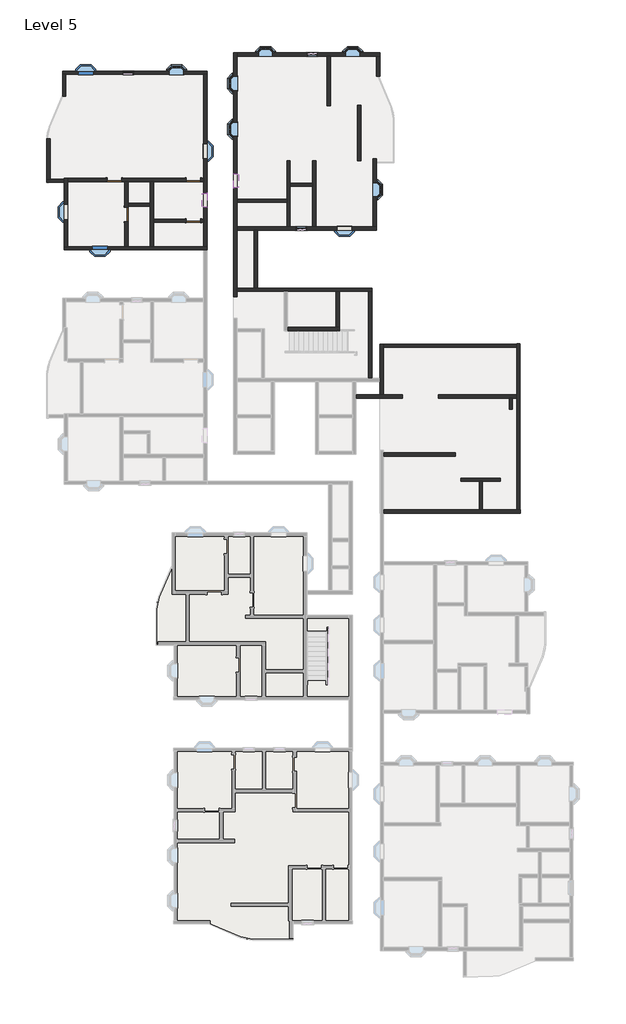
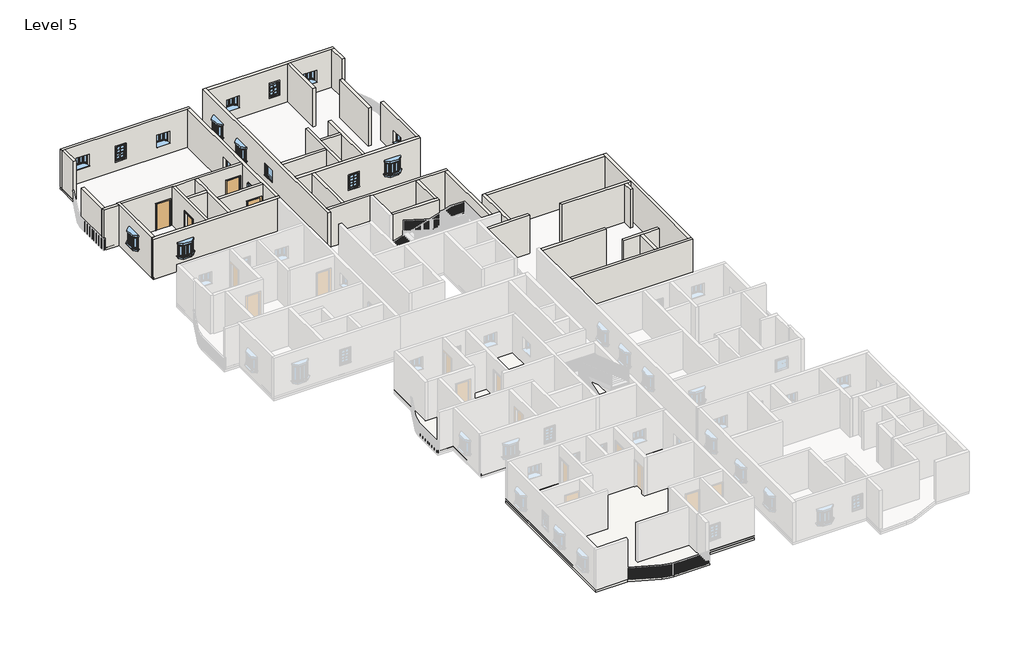
# One storey, part 4 of 14: 38 walls, 16 windows, 4 doors, 2 roofs, 1 slab.
"""IFC4 building model written with IfcOpenShell, lengths in millimetres."""

from ifc_helpers import new_model, si_unit, point, frame, frame_2d, origin, place, context, project, spatial, polyline, circle_curve, trimmed, segment, composite_curve, outline, extrude, faceted_brep, transform, mapped, element, save
from components import door_719f80de, window_910x910mm_67ef725a, window_8debb0fa, windows_sgl_w_glazing_bars_910x910mm_256712d0

model = new_model("IFC4")

# Units and contexts
model_context = context("Model", 3, world=origin())
ifc_project = project(units=[si_unit("LENGTHUNIT", "METRE", prefix="MILLI")], contexts=[model_context])

# Site, building, storey
site = spatial("IfcSite", under=ifc_project)
building = spatial("IfcBuilding", under=site)
storey = spatial("IfcBuildingStorey", under=building, Name="Level 5", Elevation=12192.0)

# Doors
placement = place(None, origin())
door_shape = door_719f80de(model_context)
element("IfcDoor", 1, ObjectType="Single-Flush : 36\" x 84\"", at=placement, inside=storey, context=model_context, shape_type="MappedRepresentation", body=[
    mapped(door_shape, transform((-16068.1391351, 22048.4083494, 12192.0), x_axis=(1.0, 0.0, 0.0), y_axis=(0.0, 1.0, 0.0), z_axis=(0.0, 0.0, 1.0))),
])
element("IfcDoor", 2, ObjectType="Single-Flush : 36\" x 84\"", at=placement, inside=storey, context=model_context, shape_type="MappedRepresentation", body=[
    mapped(door_shape, transform((-15306.1391351, 19864.0083494, 12192.0), x_axis=(0.0, 1.0, 0.0), y_axis=(-1.0, 0.0, 0.0), z_axis=(0.0, 0.0, 1.0))),
])
element("IfcDoor", 3, ObjectType="Single-Flush : 36\" x 84\"", at=placement, inside=storey, context=model_context, shape_type="MappedRepresentation", body=[
    mapped(door_shape, transform((-11057.9891351, 19470.3083494, 12192.0), x_axis=(1.0, 0.0, 0.0), y_axis=(0.0, 1.0, 0.0), z_axis=(0.0, 0.0, 1.0))),
])
element("IfcDoor", 4, ObjectType="Single-Flush : 36\" x 84\"", at=placement, inside=storey, context=model_context, shape_type="MappedRepresentation", body=[
    mapped(door_shape, transform((-11057.9891351, 22048.4083494, 12192.0), x_axis=(1.0, 0.0, 0.0), y_axis=(0.0, 1.0, 0.0), z_axis=(0.0, 0.0, 1.0))),
])

# Roofs
element("IfcRoof", 5, ObjectType="Generic - 12\"", at=placement, inside=storey, context=model_context, shape_type="SweptSolid", body=[
    extrude(outline(composite_curve([segment(polyline([(-10024.8708389, -25100.3416506), (-12290.487215, -25100.3416506), (-12290.487215, -13962.4416506), (-986.8891351, -13962.4416506), (-986.8891351, -25100.3416506), (-4746.0891351, -25100.3416506), (-4746.0891351, -26090.9416506), (-7315.6413127, -26090.9416506)]), True, "CONTINUOUS"), segment(trimmed(circle_curve(frame_2d((-7315.6413127, -24160.5416506)), 1930.4), [point((-7315.6413127, -26090.9416506))], [point((-8075.5356374, -25935.0851906))], False, "CARTESIAN"), True, "CONTINUOUS"), segment(polyline([(-8075.5356374, -25935.0851906), (-10024.8708389, -25100.3416506)]), True, "CONTINUOUS")], self_intersect=False)), frame((0.0, 0.0, 12192.0), z_axis=(0.0, 0.0, 1.0), x_axis=(1.0, 0.0, 0.0)), (0.0, 0.0, 1.0), 152.4),
])
element("IfcRoof", 6, ObjectType="Generic - 12\"", at=placement, inside=storey, context=model_context, shape_type="SweptSolid", body=[
    extrude(outline(composite_curve([segment(polyline([(-13395.387215, -7421.9416506), (-13395.387215, -5140.4900045)]), True, "CONTINUOUS"), segment(trimmed(circle_curve(frame_2d((-11464.987215, -5140.4900045)), 1930.4), [point((-13395.387215, -5140.4900045))], [point((-13239.530755, -4380.5956799))], False, "CARTESIAN"), True, "CONTINUOUS"), segment(polyline([(-13239.530755, -4380.5956799), (-12404.787215, -2431.2604783), (-12404.787215, -322.6416506), (-3857.687215, -322.6416506), (-3857.687215, -5523.2916506), (-974.1891351, -5523.2916506), (-974.1891351, -10889.0416506), (-12290.487215, -10889.0416506), (-12290.487215, -7421.9416506), (-13395.387215, -7421.9416506)]), True, "CONTINUOUS")], self_intersect=False)), frame((0.0, 0.0, 12192.0), z_axis=(0.0, 0.0, 1.0), x_axis=(1.0, 0.0, 0.0)), (0.0, 0.0, 1.0), 152.4),
])

# Slab
element("IfcSlab", 7, ObjectType="Generic - 12\"", at=placement, inside=storey, context=model_context, shape_type="SweptSolid", body=[
    extrude(outline(composite_curve([segment(polyline([(-10024.8708389, -25100.3416506), (-12290.487215, -25100.3416506), (-12290.487215, -13962.4416506), (-986.8891351, -13962.4416506), (-986.8891351, -25100.3416506), (-4746.0891351, -25100.3416506), (-4746.0891351, -26090.9416506), (-7315.6413127, -26090.9416506)]), True, "CONTINUOUS"), segment(trimmed(circle_curve(frame_2d((-7315.6413127, -24160.5416506)), 1930.4), [point((-7315.6413127, -26090.9416506))], [point((-8075.5356374, -25935.0851906))], False, "CARTESIAN"), True, "CONTINUOUS"), segment(polyline([(-8075.5356374, -25935.0851906), (-10024.8708389, -25100.3416506)]), True, "CONTINUOUS")], self_intersect=False)), frame((0.0, 0.0, 12039.6), z_axis=(0.0, 0.0, 1.0), x_axis=(1.0, 0.0, 0.0)), (0.0, 0.0, 1.0), 152.4),
])

# Walls
element("IfcWall", 8, ObjectType="4.5\" p", at=placement, inside=storey, context=model_context, shape_type="Brep", body=[
    faceted_brep([(-10600.7891351, 21946.8083494, 14325.6), (-10600.7891351, 21946.8083494, 12192.0), (-10397.5891351, 21946.8083494, 12192.0), (-10397.5891351, 21946.8083494, 15240.0), (-13578.9391351, 21946.8083494, 15240.0), (-13782.1391351, 21946.8083494, 15240.0), (-15204.5391351, 21946.8083494, 15240.0), (-15407.7391351, 21946.8083494, 15240.0), (-19033.5891351, 21946.8083494, 15240.0), (-19033.5891351, 21946.8083494, 12192.0), (-16525.3391351, 21946.8083494, 12192.0), (-16525.3391351, 21946.8083494, 14325.6), (-15610.9391351, 21946.8083494, 14325.6), (-15610.9391351, 21946.8083494, 12192.0), (-15407.7391351, 21946.8083494, 12192.0), (-15204.5391351, 21946.8083494, 12192.0), (-13782.1391351, 21946.8083494, 12192.0), (-13578.9391351, 21946.8083494, 12192.0), (-11515.1891351, 21946.8083494, 12192.0), (-11515.1891351, 21946.8083494, 14325.6), (-10397.5891351, 22150.0083494, 12192.0), (-10600.7891351, 22150.0083494, 12192.0), (-10600.7891351, 22150.0083494, 14325.6), (-11515.1891351, 22150.0083494, 14325.6), (-11515.1891351, 22150.0083494, 12192.0), (-15610.9391351, 22150.0083494, 12192.0), (-15610.9391351, 22150.0083494, 14325.6), (-16525.3391351, 22150.0083494, 14325.6), (-16525.3391351, 22150.0083494, 12192.0), (-19033.5891351, 22150.0083494, 12192.0), (-19033.5891351, 22150.0083494, 15240.0), (-10397.5891351, 22150.0083494, 15240.0)], [[[0, 1, 2, 3, 4, 5, 6, 7, 8, 9, 10, 11, 12, 13, 14, 15, 16, 17, 18, 19]], [[20, 21, 22, 23, 24, 25, 26, 27, 28, 29, 30, 31]], [[10, 9, 29, 28]], [[2, 1, 21, 20]], [[18, 17, 16, 15, 14, 13, 25, 24]], [[8, 7, 6, 5, 4, 3, 31, 30]], [[9, 8, 30, 29]], [[26, 25, 13, 12]], [[27, 26, 12, 11]], [[28, 27, 11, 10]], [[22, 21, 1, 0]], [[23, 22, 0, 19]], [[24, 23, 19, 18]], [[3, 2, 20, 31]]]),
])
element("IfcWall", 9, ObjectType="4.5\" p", at=placement, inside=storey, context=model_context, shape_type="Brep", body=[
    faceted_brep([(-15407.7391351, 21946.8083494, 12192.0), (-15407.7391351, 20321.2083494, 12192.0), (-15407.7391351, 20321.2083494, 14325.6), (-15407.7391351, 19406.8083494, 14325.6), (-15407.7391351, 19406.8083494, 12192.0), (-15407.7391351, 17812.9583494, 12192.0), (-15407.7391351, 17812.9583494, 15240.0), (-15407.7391351, 21946.8083494, 15240.0), (-15204.5391351, 20321.2083494, 14325.6), (-15204.5391351, 20321.2083494, 12192.0), (-15204.5391351, 20372.0083494, 12192.0), (-15204.5391351, 20575.2083494, 12192.0), (-15204.5391351, 21946.8083494, 12192.0), (-15204.5391351, 21946.8083494, 15240.0), (-15204.5391351, 20575.2083494, 15240.0), (-15204.5391351, 20372.0083494, 15240.0), (-15204.5391351, 17812.9583494, 15240.0), (-15204.5391351, 17812.9583494, 12192.0), (-15204.5391351, 19406.8083494, 12192.0), (-15204.5391351, 19406.8083494, 14325.6)], [[[0, 1, 2, 3, 4, 5, 6, 7]], [[8, 9, 10, 11, 12, 13, 14, 15, 16, 17, 18, 19]], [[18, 17, 5, 4]], [[12, 11, 10, 9, 1, 0]], [[7, 6, 16, 15, 14, 13]], [[6, 5, 17, 16]], [[0, 7, 13, 12]], [[2, 1, 9, 8]], [[3, 2, 8, 19]], [[4, 3, 19, 18]]]),
])
element("IfcWall", 10, ObjectType="4.5\" p", at=placement, inside=storey, context=model_context, shape_type="Brep", body=[
    faceted_brep([(-13782.1391351, 21946.8083494, 12192.0), (-13782.1391351, 20575.2083494, 12192.0), (-13782.1391351, 20372.0083494, 12192.0), (-13782.1391351, 17812.9583494, 12192.0), (-13782.1391351, 17812.9583494, 15240.0), (-13782.1391351, 20372.0083494, 15240.0), (-13782.1391351, 20575.2083494, 15240.0), (-13782.1391351, 21946.8083494, 15240.0), (-13578.9391351, 21946.8083494, 12192.0), (-13578.9391351, 21946.8083494, 15240.0), (-13578.9391351, 19571.9083494, 15240.0), (-13578.9391351, 19368.7083494, 15240.0), (-13578.9391351, 17812.9583494, 15240.0), (-13578.9391351, 17812.9583494, 12192.0), (-13578.9391351, 19368.7083494, 12192.0), (-13578.9391351, 19571.9083494, 12192.0)], [[[0, 1, 2, 3, 4, 5, 6, 7]], [[8, 9, 10, 11, 12, 13, 14, 15]], [[3, 2, 1, 0, 8, 15, 14, 13]], [[7, 6, 5, 4, 12, 11, 10, 9]], [[4, 3, 13, 12]], [[0, 7, 9, 8]]]),
])
element("IfcWall", 11, ObjectType="4.5\" p", at=placement, inside=storey, context=model_context, shape_type="SweptSolid", body=[
    extrude(outline(polyline([(-13782.1391351, 20372.0083494), (-15204.5391351, 20372.0083494), (-15204.5391351, 20575.2083494), (-13782.1391351, 20575.2083494), (-13782.1391351, 20372.0083494)])), frame((0.0, 0.0, 12192.0), z_axis=(0.0, 0.0, 1.0), x_axis=(1.0, 0.0, 0.0)), (0.0, 0.0, 1.0), 3048.0),
])
element("IfcWall", 12, ObjectType="4.5\" p", at=placement, inside=storey, context=model_context, shape_type="SweptSolid", body=[
    extrude(outline(polyline([(14325.6, -10600.7891351), (12192.0, -10600.7891351), (12192.0, -10397.5891351), (15240.0, -10397.5891351), (15240.0, -13578.9391351), (12192.0, -13578.9391351), (12192.0, -11515.1891351), (14325.6, -11515.1891351), (14325.6, -10600.7891351)])), frame((0.0, 19368.7083494, 0.0), z_axis=(0.0, 1.0, 0.0), x_axis=(0.0, 0.0, 1.0)), (0.0, 0.0, 1.0), 203.2),
])
element("IfcWall", 13, ObjectType="4.5\" p", at=placement, inside=storey, context=model_context, shape_type="SweptSolid", body=[
    extrude(outline(polyline([(-6993.9891351, 18875.1215905), (-6993.9891351, 15192.1215905), (-7197.1891351, 15192.1215905), (-7197.1891351, 18875.1215905), (-6993.9891351, 18875.1215905)])), frame((0.0, 0.0, 12192.0), z_axis=(0.0, 0.0, 1.0), x_axis=(1.0, 0.0, 0.0)), (0.0, 0.0, 1.0), 3048.0),
])
element("IfcWall", 14, ObjectType="4.5\" p", at=placement, inside=storey, context=model_context, shape_type="Brep", body=[
    faceted_brep([(-8289.3891351, 18875.1215905, 12192.0), (-7197.1891351, 18875.1215905, 12192.0), (-6993.9891351, 18875.1215905, 12192.0), (562.5108649, 18875.1215905, 12192.0), (562.5108649, 18875.1215905, 15240.0), (-6993.9891351, 18875.1215905, 15240.0), (-7197.1891351, 18875.1215905, 15240.0), (-8289.3891351, 18875.1215905, 15240.0), (-1017.6641351, 18875.1215905, 14302.0), (-1017.6641351, 18875.1215905, 13392.0), (-1927.6641351, 18875.1215905, 13392.0), (-1927.6641351, 18875.1215905, 14302.0), (-3876.1391351, 18875.1215905, 14173.2), (-3876.1391351, 18875.1215905, 13106.4), (-4536.5391351, 18875.1215905, 13106.4), (-4536.5391351, 18875.1215905, 14173.2), (-8289.3891351, 19078.3215905, 12192.0), (-8289.3891351, 19078.3215905, 15240.0), (-5120.7391351, 19078.3215905, 15240.0), (-4917.5391351, 19078.3215905, 15240.0), (-3495.1391351, 19078.3215905, 15240.0), (-3291.9391351, 19078.3215905, 15240.0), (346.6108649, 19078.3215905, 15240.0), (549.8108649, 19078.3215905, 15240.0), (562.5108649, 19078.3215905, 15240.0), (562.5108649, 19078.3215905, 12192.0), (549.8108649, 19078.3215905, 12192.0), (346.6108649, 19078.3215905, 12192.0), (-3291.9391351, 19078.3215905, 12192.0), (-3495.1391351, 19078.3215905, 12192.0), (-4917.5391351, 19078.3215905, 12192.0), (-5120.7391351, 19078.3215905, 12192.0), (-1017.6641351, 19078.3215905, 14302.0), (-1927.6641351, 19078.3215905, 14302.0), (-1927.6641351, 19078.3215905, 13392.0), (-1017.6641351, 19078.3215905, 13392.0), (-3876.1391351, 19078.3215905, 14173.2), (-4536.5391351, 19078.3215905, 14173.2), (-4536.5391351, 19078.3215905, 13106.4), (-3876.1391351, 19078.3215905, 13106.4)], [[[0, 1, 2, 3, 4, 5, 6, 7], [8, 9, 10, 11], [12, 13, 14, 15]], [[16, 17, 18, 19, 20, 21, 22, 23, 24, 25, 26, 27, 28, 29, 30, 31], [32, 33, 34, 35], [36, 37, 38, 39]], [[3, 2, 1, 0, 16, 31, 30, 29, 28, 27, 26, 25]], [[4, 3, 25, 24]], [[7, 6, 5, 4, 24, 23, 22, 21, 20, 19, 18, 17]], [[9, 8, 32, 35]], [[10, 9, 35, 34]], [[11, 10, 34, 33]], [[8, 11, 33, 32]], [[13, 12, 36, 39]], [[14, 13, 39, 38]], [[15, 14, 38, 37]], [[12, 15, 37, 36]], [[0, 7, 17, 16]]]),
])
element("IfcWall", 15, ObjectType="4.5\" p", at=placement, inside=storey, context=model_context, shape_type="SweptSolid", body=[
    extrude(outline(polyline([(19078.3215905, 12192.0), (19078.3215905, 15240.0), (23396.3215905, 15240.0), (23396.3215905, 12192.0), (19078.3215905, 12192.0)]), holes=[polyline([(21882.8215905, 14016.4), (20972.8215905, 14016.4), (20972.8215905, 13106.4), (21882.8215905, 13106.4), (21882.8215905, 14016.4)])]), frame((346.6108649, 0.0, 0.0), z_axis=(1.0, 0.0, 0.0), x_axis=(0.0, 1.0, 0.0)), (0.0, 0.0, 1.0), 203.2),
])
element("IfcWall", 16, ObjectType="4.5\" p", at=placement, inside=storey, context=model_context, shape_type="SweptSolid", body=[
    extrude(outline(polyline([(-5120.7391351, 20634.0715905), (-8289.3891351, 20634.0715905), (-8289.3891351, 20837.2715905), (-5120.7391351, 20837.2715905), (-5120.7391351, 20634.0715905)])), frame((0.0, 0.0, 12192.0), z_axis=(0.0, 0.0, 1.0), x_axis=(1.0, 0.0, 0.0)), (0.0, 0.0, 1.0), 3048.0),
])
element("IfcWall", 17, ObjectType="4.5\" p", at=placement, inside=storey, context=model_context, shape_type="Brep", body=[
    faceted_brep([(-5120.7391351, 23256.6215905, 12192.0), (-5120.7391351, 20837.2715905, 12192.0), (-5120.7391351, 20634.0715905, 12192.0), (-5120.7391351, 19078.3215905, 12192.0), (-5120.7391351, 19078.3215905, 15240.0), (-5120.7391351, 20634.0715905, 15240.0), (-5120.7391351, 20837.2715905, 15240.0), (-5120.7391351, 23256.6215905, 15240.0), (-4917.5391351, 23256.6215905, 12192.0), (-4917.5391351, 23256.6215905, 15240.0), (-4917.5391351, 21853.2715905, 15240.0), (-4917.5391351, 21650.0715905, 15240.0), (-4917.5391351, 19078.3215905, 15240.0), (-4917.5391351, 19078.3215905, 12192.0), (-4917.5391351, 21650.0715905, 12192.0), (-4917.5391351, 21853.2715905, 12192.0)], [[[0, 1, 2, 3, 4, 5, 6, 7]], [[8, 9, 10, 11, 12, 13, 14, 15]], [[3, 2, 1, 0, 8, 15, 14, 13]], [[7, 6, 5, 4, 12, 11, 10, 9]], [[0, 7, 9, 8]], [[4, 3, 13, 12]]]),
])
element("IfcWall", 18, ObjectType="4.5\" p", at=placement, inside=storey, context=model_context, shape_type="Brep", body=[
    faceted_brep([(-3495.1391351, 23256.6215905, 12192.0), (-3495.1391351, 21853.2715905, 12192.0), (-3495.1391351, 21650.0715905, 12192.0), (-3495.1391351, 19078.3215905, 12192.0), (-3495.1391351, 19078.3215905, 15240.0), (-3495.1391351, 21650.0715905, 15240.0), (-3495.1391351, 21853.2715905, 15240.0), (-3495.1391351, 23256.6215905, 15240.0), (-3291.9391351, 23256.6215905, 12192.0), (-3291.9391351, 23256.6215905, 15240.0), (-3291.9391351, 19078.3215905, 15240.0), (-3291.9391351, 19078.3215905, 12192.0)], [[[0, 1, 2, 3, 4, 5, 6, 7]], [[8, 9, 10, 11]], [[3, 2, 1, 0, 8, 11]], [[7, 6, 5, 4, 10, 9]], [[0, 7, 9, 8]], [[4, 3, 11, 10]]]),
])
element("IfcWall", 19, ObjectType="4.5\" p", at=placement, inside=storey, context=model_context, shape_type="SweptSolid", body=[
    extrude(outline(polyline([(-3495.1391351, 21650.0715905), (-4917.5391351, 21650.0715905), (-4917.5391351, 21853.2715905), (-3495.1391351, 21853.2715905), (-3495.1391351, 21650.0715905)])), frame((0.0, 0.0, 12192.0), z_axis=(0.0, 0.0, 1.0), x_axis=(1.0, 0.0, 0.0)), (0.0, 0.0, 1.0), 3048.0),
])
element("IfcWall", 20, ObjectType="4.5\" p", at=placement, inside=storey, context=model_context, shape_type="SweptSolid", body=[
    extrude(outline(polyline([(-1799.6891351, 14988.9215905), (-1799.6891351, 12709.2715905), (-2002.8891351, 12709.2715905), (-2002.8891351, 14988.9215905), (-1799.6891351, 14988.9215905)])), frame((0.0, 0.0, 12192.0), z_axis=(0.0, 0.0, 1.0), x_axis=(1.0, 0.0, 0.0)), (0.0, 0.0, 1.0), 3048.0),
])
element("IfcWall", 21, ObjectType="4.5\" p", at=placement, inside=storey, context=model_context, shape_type="Brep", body=[
    faceted_brep([(-5095.3391351, 12506.0715905, 12192.0), (-1786.9891351, 12506.0715905, 12192.0), (-1786.9891351, 12506.0715905, 15240.0), (-5095.3391351, 12506.0715905, 15240.0), (-5095.3391351, 12709.2715905, 12192.0), (-5095.3391351, 12709.2715905, 15240.0), (-2002.8891351, 12709.2715905, 15240.0), (-1799.6891351, 12709.2715905, 15240.0), (-1786.9891351, 12709.2715905, 15240.0), (-1786.9891351, 12709.2715905, 12192.0), (-1799.6891351, 12709.2715905, 12192.0), (-2002.8891351, 12709.2715905, 12192.0)], [[[0, 1, 2, 3]], [[4, 5, 6, 7, 8, 9, 10, 11]], [[1, 0, 4, 11, 10, 9]], [[2, 1, 9, 8]], [[3, 2, 8, 7, 6, 5]], [[0, 3, 5, 4]]]),
])
element("IfcWall", 22, ObjectType="4.5\" p", at=placement, inside=storey, context=model_context, shape_type="Brep", body=[
    faceted_brep([(-745.5891351, 8223.6457306, 12192.0), (2209.4205024, 8223.6457306, 12192.0), (2209.4205024, 8223.6457306, 15240.0), (-745.5891351, 8223.6457306, 15240.0), (-745.5891351, 8426.8457306, 12192.0), (-745.5891351, 8426.8457306, 15240.0), (793.5880523, 8426.8457306, 15240.0), (996.7880523, 8426.8457306, 15240.0), (2209.4205024, 8426.8457306, 15240.0), (2209.4205024, 8426.8457306, 12192.0), (996.7880523, 8426.8457306, 12192.0), (793.5880523, 8426.8457306, 12192.0)], [[[0, 1, 2, 3]], [[4, 5, 6, 7, 8, 9, 10, 11]], [[1, 0, 4, 11, 10, 9]], [[2, 1, 9, 8]], [[3, 2, 8, 7, 6, 5]], [[0, 3, 5, 4]]]),
])
element("IfcWall", 23, ObjectType="4.5\" p", at=placement, inside=storey, context=model_context, shape_type="Brep", body=[
    faceted_brep([(996.7880523, 8426.8457306, 12192.0), (996.7880523, 11443.0957306, 12192.0), (996.7880523, 11646.2957306, 12192.0), (996.7880523, 11646.2957306, 15240.0), (996.7880523, 11443.0957306, 15240.0), (996.7880523, 8426.8457306, 15240.0), (793.5880523, 8426.8457306, 12192.0), (793.5880523, 8426.8457306, 15240.0), (793.5880523, 9275.2949943, 15240.0), (793.5880523, 9478.4949943, 15240.0), (793.5880523, 11646.2957306, 15240.0), (793.5880523, 11646.2957306, 12192.0), (793.5880523, 9478.4949943, 12192.0), (793.5880523, 9275.2949943, 12192.0)], [[[0, 1, 2, 3, 4, 5]], [[6, 7, 8, 9, 10, 11, 12, 13]], [[2, 1, 0, 6, 13, 12, 11]], [[5, 4, 3, 10, 9, 8, 7]], [[0, 5, 7, 6]], [[3, 2, 11, 10]]]),
])
element("IfcWall", 24, ObjectType="4.5\" p", at=placement, inside=storey, context=model_context, shape_type="Brep", body=[
    faceted_brep([(9461.3380523, 8426.8457306, 12192.0), (4492.3034266, 8426.8457306, 12192.0), (4492.3034266, 8426.8457306, 15240.0), (9461.3380523, 8426.8457306, 15240.0), (9461.3380523, 8223.6457306, 12192.0), (9461.3380523, 8223.6457306, 15240.0), (9181.9380523, 8223.6457306, 15240.0), (8978.7380523, 8223.6457306, 15240.0), (4492.3034266, 8223.6457306, 15240.0), (4492.3034266, 8223.6457306, 12192.0), (8978.7380523, 8223.6457306, 12192.0), (9181.9380523, 8223.6457306, 12192.0)], [[[0, 1, 2, 3]], [[4, 5, 6, 7, 8, 9, 10, 11]], [[1, 0, 4, 11, 10, 9]], [[2, 1, 9, 8]], [[3, 2, 8, 7, 6, 5]], [[0, 3, 5, 4]]]),
])
element("IfcWall", 25, ObjectType="4.5\" p", at=placement, inside=storey, context=model_context, shape_type="Brep", body=[
    faceted_brep([(1007.0108649, 940.1957306, 12192.0), (9677.2380523, 940.1957306, 12192.0), (9677.2380523, 940.1957306, 15240.0), (1007.0108649, 940.1957306, 15240.0), (1007.0108649, 1143.3957306, 12192.0), (1007.0108649, 1143.3957306, 15240.0), (7073.7380523, 1143.3957306, 15240.0), (7276.9380523, 1143.3957306, 15240.0), (9461.3380523, 1143.3957306, 15240.0), (9664.5380523, 1143.3957306, 15240.0), (9677.2380523, 1143.3957306, 15240.0), (9677.2380523, 1143.3957306, 12192.0), (9664.5380523, 1143.3957306, 12192.0), (9461.3380523, 1143.3957306, 12192.0), (7276.9380523, 1143.3957306, 12192.0), (7073.7380523, 1143.3957306, 12192.0)], [[[0, 1, 2, 3]], [[4, 5, 6, 7, 8, 9, 10, 11, 12, 13, 14, 15]], [[1, 0, 4, 15, 14, 13, 12, 11]], [[2, 1, 11, 10]], [[3, 2, 10, 9, 8, 7, 6, 5]], [[0, 3, 5, 4]]]),
])
element("IfcWall", 26, ObjectType="4.5\" p", at=placement, inside=storey, context=model_context, shape_type="Brep", body=[
    faceted_brep([(9664.5380523, 1143.3957306, 12192.0), (9664.5380523, 11658.9957306, 12192.0), (9664.5380523, 11658.9957306, 15240.0), (9664.5380523, 1143.3957306, 15240.0), (9461.3380523, 1143.3957306, 12192.0), (9461.3380523, 1143.3957306, 15240.0), (9461.3380523, 8223.6457306, 15240.0), (9461.3380523, 8426.8457306, 15240.0), (9461.3380523, 11443.0957306, 15240.0), (9461.3380523, 11646.2957306, 15240.0), (9461.3380523, 11658.9957306, 15240.0), (9461.3380523, 11658.9957306, 12192.0), (9461.3380523, 11646.2957306, 12192.0), (9461.3380523, 11443.0957306, 12192.0), (9461.3380523, 8426.8457306, 12192.0), (9461.3380523, 8223.6457306, 12192.0)], [[[0, 1, 2, 3]], [[4, 5, 6, 7, 8, 9, 10, 11, 12, 13, 14, 15]], [[1, 0, 4, 15, 14, 13, 12, 11]], [[2, 1, 11, 10]], [[3, 2, 10, 9, 8, 7, 6, 5]], [[0, 3, 5, 4]]]),
])
element("IfcWall", 27, ObjectType="4.5\" p", at=placement, inside=storey, context=model_context, shape_type="SweptSolid", body=[
    extrude(outline(polyline([(-643.9891351, 23256.6215905), (-643.9891351, 26780.8715905), (-440.7891351, 26780.8715905), (-440.7891351, 23256.6215905), (-643.9891351, 23256.6215905)])), frame((0.0, 0.0, 12192.0), z_axis=(0.0, 0.0, 1.0), x_axis=(1.0, 0.0, 0.0)), (0.0, 0.0, 1.0), 3048.0),
])
element("IfcWall", 28, ObjectType="4.5\" p", at=placement, inside=storey, context=model_context, shape_type="SweptSolid", body=[
    extrude(outline(polyline([(-2568.0391351, 26760.9286213), (-2568.0391351, 29898.7215905), (-2364.8391351, 29898.7215905), (-2364.8391351, 26760.9286213), (-2568.0391351, 26760.9286213)])), frame((0.0, 0.0, 12192.0), z_axis=(0.0, 0.0, 1.0), x_axis=(1.0, 0.0, 0.0)), (0.0, 0.0, 1.0), 3048.0),
])
element("IfcWall", 29, ObjectType="4.5\" p", at=placement, inside=storey, context=model_context, shape_type="SweptSolid", body=[
    extrude(outline(polyline([(765.7108649, 29898.7215905), (765.7108649, 28631.1875845), (562.5108649, 28631.1875845), (562.5108649, 29898.7215905), (765.7108649, 29898.7215905)])), frame((0.0, 0.0, 12192.0), z_axis=(0.0, 0.0, 1.0), x_axis=(1.0, 0.0, 0.0)), (0.0, 0.0, 1.0), 3048.0),
])
element("IfcWall", 30, ObjectType="9\" w", at=placement, inside=storey, context=model_context, shape_type="Brep", body=[
    faceted_brep([(-10181.6891351, 17812.9583494, 12192.0), (-10194.3891351, 17812.9583494, 12192.0), (-10397.5891351, 17812.9583494, 12192.0), (-13578.9391351, 17812.9583494, 12192.0), (-13782.1391351, 17812.9583494, 12192.0), (-15204.5391351, 17812.9583494, 12192.0), (-15407.7391351, 17812.9583494, 12192.0), (-19033.5891351, 17812.9583494, 12192.0), (-19236.7891351, 17812.9583494, 12192.0), (-19249.4891351, 17812.9583494, 12192.0), (-19249.4891351, 17812.9583494, 15240.0), (-19236.7891351, 17812.9583494, 15240.0), (-19033.5891351, 17812.9583494, 15240.0), (-15407.7391351, 17812.9583494, 15240.0), (-15204.5391351, 17812.9583494, 15240.0), (-13782.1391351, 17812.9583494, 15240.0), (-13578.9391351, 17812.9583494, 15240.0), (-10397.5891351, 17812.9583494, 15240.0), (-10194.3891351, 17812.9583494, 15240.0), (-10181.6891351, 17812.9583494, 15240.0), (-16527.5391351, 17812.9583494, 14302.0), (-17437.5391351, 17812.9583494, 14302.0), (-17437.5391351, 17812.9583494, 13392.0), (-16527.5391351, 17812.9583494, 13392.0), (-10181.6891351, 17609.7583494, 12192.0), (-10181.6891351, 17609.7583494, 15240.0), (-19249.4891351, 17609.7583494, 15240.0), (-19249.4891351, 17609.7583494, 12192.0), (-16527.5391351, 17609.7583494, 14302.0), (-16527.5391351, 17609.7583494, 13392.0), (-17437.5391351, 17609.7583494, 13392.0), (-17437.5391351, 17609.7583494, 14302.0)], [[[0, 1, 2, 3, 4, 5, 6, 7, 8, 9, 10, 11, 12, 13, 14, 15, 16, 17, 18, 19], [20, 21, 22, 23]], [[24, 25, 26, 27], [28, 29, 30, 31]], [[9, 8, 7, 6, 5, 4, 3, 2, 1, 0, 24, 27]], [[10, 9, 27, 26]], [[19, 18, 17, 16, 15, 14, 13, 12, 11, 10, 26, 25]], [[0, 19, 25, 24]], [[29, 28, 20, 23]], [[30, 29, 23, 22]], [[31, 30, 22, 21]], [[28, 31, 21, 20]]]),
])
element("IfcWall", 31, ObjectType="9\" w", at=placement, inside=storey, context=model_context, shape_type="Brep", body=[
    faceted_brep([(-19033.5891351, 17812.9583494, 12192.0), (-19033.5891351, 21946.8083494, 12192.0), (-19033.5891351, 22150.0083494, 12192.0), (-19033.5891351, 22150.0083494, 15240.0), (-19033.5891351, 21946.8083494, 15240.0), (-19033.5891351, 17812.9583494, 15240.0), (-19033.5891351, 19555.0583494, 14302.0), (-19033.5891351, 20465.0583494, 14302.0), (-19033.5891351, 20465.0583494, 13392.0), (-19033.5891351, 19555.0583494, 13392.0), (-19236.7891351, 17812.9583494, 12192.0), (-19236.7891351, 17812.9583494, 15240.0), (-19236.7891351, 21889.6583494, 15240.0), (-19236.7891351, 22092.8583494, 15240.0), (-19236.7891351, 22150.0083494, 15240.0), (-19236.7891351, 22150.0083494, 12192.0), (-19236.7891351, 22092.8583494, 12192.0), (-19236.7891351, 21889.6583494, 12192.0), (-19236.7891351, 19555.0583494, 14302.0), (-19236.7891351, 19555.0583494, 13392.0), (-19236.7891351, 20465.0583494, 13392.0), (-19236.7891351, 20465.0583494, 14302.0)], [[[0, 1, 2, 3, 4, 5], [6, 7, 8, 9]], [[10, 11, 12, 13, 14, 15, 16, 17], [18, 19, 20, 21]], [[2, 1, 0, 10, 17, 16, 15]], [[5, 4, 3, 14, 13, 12, 11]], [[0, 5, 11, 10]], [[3, 2, 15, 14]], [[19, 18, 6, 9]], [[20, 19, 9, 8]], [[21, 20, 8, 7]], [[18, 21, 7, 6]]]),
])
element("IfcWall", 32, ObjectType="9\" w", at=placement, inside=storey, context=model_context, shape_type="Brep", body=[
    faceted_brep([(-20341.6891351, 21889.6583494, 12192.0), (-19236.7891351, 21889.6583494, 12192.0), (-19236.7891351, 21889.6583494, 15240.0), (-20341.6891351, 21889.6583494, 15240.0), (-20341.6891351, 22092.8583494, 12192.0), (-20341.6891351, 22092.8583494, 15240.0), (-20138.4891351, 22092.8583494, 15240.0), (-19236.7891351, 22092.8583494, 15240.0), (-19236.7891351, 22092.8583494, 12192.0), (-20138.4891351, 22092.8583494, 12192.0)], [[[0, 1, 2, 3]], [[4, 5, 6, 7, 8, 9]], [[1, 0, 4, 9, 8]], [[3, 2, 7, 6, 5]], [[0, 3, 5, 4]], [[2, 1, 8, 7]]]),
])
element("IfcWall", 33, ObjectType="9\" w", at=placement, inside=storey, context=model_context, shape_type="SweptSolid", body=[
    extrude(outline(polyline([(-20341.6891351, 22092.8583494), (-20341.6891351, 24656.5948172), (-20138.4891351, 24656.5948172), (-20138.4891351, 22092.8583494), (-20341.6891351, 22092.8583494)])), frame((0.0, 0.0, 12192.0), z_axis=(0.0, 0.0, 1.0), x_axis=(1.0, 0.0, 0.0)), (0.0, 0.0, 1.0), 3048.0),
])
element("IfcWall", 34, ObjectType="9\" w", at=placement, inside=storey, context=model_context, shape_type="Brep", body=[
    faceted_brep([(-8289.3891351, 14988.9215905, 12192.0), (-5298.5391351, 14988.9215905, 12192.0), (-5095.3391351, 14988.9215905, 12192.0), (-2002.8891351, 14988.9215905, 12192.0), (-1799.6891351, 14988.9215905, 12192.0), (54.5108649, 14988.9215905, 12192.0), (257.7108649, 14988.9215905, 12192.0), (270.4108649, 14988.9215905, 12192.0), (270.4108649, 14988.9215905, 15240.0), (257.7108649, 14988.9215905, 15240.0), (54.5108649, 14988.9215905, 15240.0), (-1799.6891351, 14988.9215905, 15240.0), (-2002.8891351, 14988.9215905, 15240.0), (-5095.3391351, 14988.9215905, 15240.0), (-5298.5391351, 14988.9215905, 15240.0), (-8289.3891351, 14988.9215905, 15240.0), (-8289.3891351, 15192.1215905, 12192.0), (-8289.3891351, 15192.1215905, 15240.0), (-7197.1891351, 15192.1215905, 15240.0), (-6993.9891351, 15192.1215905, 15240.0), (270.4108649, 15192.1215905, 15240.0), (270.4108649, 15192.1215905, 12192.0), (-6993.9891351, 15192.1215905, 12192.0), (-7197.1891351, 15192.1215905, 12192.0)], [[[0, 1, 2, 3, 4, 5, 6, 7, 8, 9, 10, 11, 12, 13, 14, 15]], [[16, 17, 18, 19, 20, 21, 22, 23]], [[7, 6, 5, 4, 3, 2, 1, 0, 16, 23, 22, 21]], [[8, 7, 21, 20]], [[15, 14, 13, 12, 11, 10, 9, 8, 20, 19, 18, 17]], [[0, 15, 17, 16]]]),
])
element("IfcWall", 35, ObjectType="9\" w", at=placement, inside=storey, context=model_context, shape_type="SweptSolid", body=[
    extrude(outline(polyline([(54.5108649, 9478.4949943), (54.5108649, 14988.9215905), (257.7108649, 14988.9215905), (257.7108649, 9478.4949943), (54.5108649, 9478.4949943)])), frame((0.0, 0.0, 12192.0), z_axis=(0.0, 0.0, 1.0), x_axis=(1.0, 0.0, 0.0)), (0.0, 0.0, 1.0), 3048.0),
])
element("IfcWall", 36, ObjectType="9\" w", at=placement, inside=storey, context=model_context, shape_type="SweptSolid", body=[
    extrude(outline(polyline([(9461.3380523, 11443.0957306), (996.7880523, 11443.0957306), (996.7880523, 11646.2957306), (9461.3380523, 11646.2957306), (9461.3380523, 11443.0957306)])), frame((0.0, 0.0, 12192.0), z_axis=(0.0, 0.0, 1.0), x_axis=(1.0, 0.0, 0.0)), (0.0, 0.0, 1.0), 3048.0),
])
element("IfcWall", 37, ObjectType="9\" w", at=placement, inside=storey, context=model_context, shape_type="SweptSolid", body=[
    extrude(outline(polyline([(8978.7380523, 7506.0957306), (8978.7380523, 8223.6457306), (9181.9380523, 8223.6457306), (9181.9380523, 7506.0957306), (8978.7380523, 7506.0957306)])), frame((0.0, 0.0, 12192.0), z_axis=(0.0, 0.0, 1.0), x_axis=(1.0, 0.0, 0.0)), (0.0, 0.0, 1.0), 3048.0),
])
element("IfcWall", 38, ObjectType="9\" w", at=placement, inside=storey, context=model_context, shape_type="SweptSolid", body=[
    extrude(outline(polyline([(7276.9380523, 2954.8622042), (7276.9380523, 1143.3957306), (7073.7380523, 1143.3957306), (7073.7380523, 2954.8622042), (7276.9380523, 2954.8622042)])), frame((0.0, 0.0, 12192.0), z_axis=(0.0, 0.0, 1.0), x_axis=(1.0, 0.0, 0.0)), (0.0, 0.0, 1.0), 3048.0),
])
element("IfcWall", 39, ObjectType="9\" w", at=placement, inside=storey, context=model_context, shape_type="Brep", body=[
    faceted_brep([(5904.1857655, 2954.8622042, 12192.0), (7073.7380523, 2954.8622042, 12192.0), (7276.9380523, 2954.8622042, 12192.0), (8418.7857655, 2954.8622042, 12192.0), (8418.7857655, 2954.8622042, 15240.0), (7276.9380523, 2954.8622042, 15240.0), (7073.7380523, 2954.8622042, 15240.0), (5904.1857655, 2954.8622042, 15240.0), (5904.1857655, 3158.0622042, 12192.0), (5904.1857655, 3158.0622042, 15240.0), (8418.7857655, 3158.0622042, 15240.0), (8418.7857655, 3158.0622042, 12192.0)], [[[0, 1, 2, 3, 4, 5, 6, 7]], [[8, 9, 10, 11]], [[3, 2, 1, 0, 8, 11]], [[4, 3, 11, 10]], [[7, 6, 5, 4, 10, 9]], [[0, 7, 9, 8]]]),
])
element("IfcWall", 40, ObjectType="9\" w", at=placement, inside=storey, context=model_context, shape_type="SweptSolid", body=[
    extrude(outline(polyline([(5571.3060189, 4550.8949943), (1007.0108649, 4550.8949943), (1007.0108649, 4754.0949943), (5571.3060189, 4754.0949943), (5571.3060189, 4550.8949943)])), frame((0.0, 0.0, 12192.0), z_axis=(0.0, 0.0, 1.0), x_axis=(1.0, 0.0, 0.0)), (0.0, 0.0, 1.0), 3048.0),
])
element("IfcWall", 41, ObjectType="9\" w", at=placement, inside=storey, context=model_context, shape_type="Brep", body=[
    faceted_brep([(-8390.9891351, 29898.7215905, 12192.0), (-2568.0391351, 29898.7215905, 12192.0), (-2364.8391351, 29898.7215905, 12192.0), (562.5108649, 29898.7215905, 12192.0), (765.7108649, 29898.7215905, 12192.0), (765.7108649, 29898.7215905, 15240.0), (562.5108649, 29898.7215905, 15240.0), (-2364.8391351, 29898.7215905, 15240.0), (-2568.0391351, 29898.7215905, 15240.0), (-8390.9891351, 29898.7215905, 15240.0), (-6931.4641351, 29898.7215905, 14016.4), (-6021.4641351, 29898.7215905, 14016.4), (-6021.4641351, 29898.7215905, 13106.4), (-6931.4641351, 29898.7215905, 13106.4), (-1406.9641351, 29898.7215905, 14016.4), (-496.9641351, 29898.7215905, 14016.4), (-496.9641351, 29898.7215905, 13106.4), (-1406.9641351, 29898.7215905, 13106.4), (-3844.3891351, 29898.7215905, 14173.2), (-3183.9891351, 29898.7215905, 14173.2), (-3183.9891351, 29898.7215905, 13106.4), (-3844.3891351, 29898.7215905, 13106.4), (-8390.9891351, 30101.9215905, 12192.0), (-8390.9891351, 30101.9215905, 15240.0), (765.7108649, 30101.9215905, 15240.0), (765.7108649, 30101.9215905, 12192.0), (-6931.4641351, 30101.9215905, 14016.4), (-6931.4641351, 30101.9215905, 13106.4), (-6021.4641351, 30101.9215905, 13106.4), (-6021.4641351, 30101.9215905, 14016.4), (-1406.9641351, 30101.9215905, 14016.4), (-1406.9641351, 30101.9215905, 13106.4), (-496.9641351, 30101.9215905, 13106.4), (-496.9641351, 30101.9215905, 14016.4), (-3844.3891351, 30101.9215905, 14173.2), (-3844.3891351, 30101.9215905, 13106.4), (-3183.9891351, 30101.9215905, 13106.4), (-3183.9891351, 30101.9215905, 14173.2)], [[[0, 1, 2, 3, 4, 5, 6, 7, 8, 9], [10, 11, 12, 13], [14, 15, 16, 17], [18, 19, 20, 21]], [[22, 23, 24, 25], [26, 27, 28, 29], [30, 31, 32, 33], [34, 35, 36, 37]], [[4, 3, 2, 1, 0, 22, 25]], [[9, 8, 7, 6, 5, 24, 23]], [[0, 9, 23, 22]], [[27, 26, 10, 13]], [[28, 27, 13, 12]], [[29, 28, 12, 11]], [[26, 29, 11, 10]], [[31, 30, 14, 17]], [[32, 31, 17, 16]], [[33, 32, 16, 15]], [[30, 33, 15, 14]], [[35, 34, 18, 21]], [[36, 35, 21, 20]], [[37, 36, 20, 19]], [[34, 37, 19, 18]], [[5, 4, 25, 24]]]),
])
element("IfcWall", 42, ObjectType="9\" w", at=placement, inside=storey, context=model_context, shape_type="Brep", body=[
    faceted_brep([(-19351.0891351, 28747.6583494, 12192.0), (-19147.8891351, 28747.6583494, 12192.0), (-10397.5891351, 28747.6583494, 12192.0), (-10194.3891351, 28747.6583494, 12192.0), (-10181.6891351, 28747.6583494, 12192.0), (-10181.6891351, 28747.6583494, 15240.0), (-10194.3891351, 28747.6583494, 15240.0), (-10397.5891351, 28747.6583494, 15240.0), (-19147.8891351, 28747.6583494, 15240.0), (-19351.0891351, 28747.6583494, 15240.0), (-18332.8891351, 28747.6583494, 14302.0), (-17422.8891351, 28747.6583494, 14302.0), (-17422.8891351, 28747.6583494, 13392.0), (-18332.8891351, 28747.6583494, 13392.0), (-12579.7891351, 28747.6583494, 14016.4), (-11669.7891351, 28747.6583494, 14016.4), (-11669.7891351, 28747.6583494, 13106.4), (-12579.7891351, 28747.6583494, 13106.4), (-14845.7641351, 28747.6583494, 14173.2), (-14845.7641351, 28747.6583494, 13106.4), (-15506.1641351, 28747.6583494, 13106.4), (-15506.1641351, 28747.6583494, 14173.2), (-19351.0891351, 28950.8583494, 12192.0), (-19351.0891351, 28950.8583494, 15240.0), (-10181.6891351, 28950.8583494, 15240.0), (-10181.6891351, 28950.8583494, 12192.0), (-18332.8891351, 28950.8583494, 14302.0), (-18332.8891351, 28950.8583494, 13392.0), (-17422.8891351, 28950.8583494, 13392.0), (-17422.8891351, 28950.8583494, 14302.0), (-12579.7891351, 28950.8583494, 14016.4), (-12579.7891351, 28950.8583494, 13106.4), (-11669.7891351, 28950.8583494, 13106.4), (-11669.7891351, 28950.8583494, 14016.4), (-14845.7641351, 28950.8583494, 14173.2), (-15506.1641351, 28950.8583494, 14173.2), (-15506.1641351, 28950.8583494, 13106.4), (-14845.7641351, 28950.8583494, 13106.4)], [[[0, 1, 2, 3, 4, 5, 6, 7, 8, 9], [10, 11, 12, 13], [14, 15, 16, 17], [18, 19, 20, 21]], [[22, 23, 24, 25], [26, 27, 28, 29], [30, 31, 32, 33], [34, 35, 36, 37]], [[4, 3, 2, 1, 0, 22, 25]], [[5, 4, 25, 24]], [[9, 8, 7, 6, 5, 24, 23]], [[27, 26, 10, 13]], [[28, 27, 13, 12]], [[29, 28, 12, 11]], [[26, 29, 11, 10]], [[31, 30, 14, 17]], [[32, 31, 17, 16]], [[33, 32, 16, 15]], [[30, 33, 15, 14]], [[19, 18, 34, 37]], [[20, 19, 37, 36]], [[21, 20, 36, 35]], [[18, 21, 35, 34]], [[0, 9, 23, 22]]]),
])
element("IfcWall", 43, ObjectType="9\" w", at=placement, inside=storey, context=model_context, shape_type="SweptSolid", body=[
    extrude(outline(polyline([(-19147.8891351, 28747.6583494), (-19147.8891351, 27344.9858981), (-19351.0891351, 27344.9858981), (-19351.0891351, 28747.6583494), (-19147.8891351, 28747.6583494)])), frame((0.0, 0.0, 12192.0), z_axis=(0.0, 0.0, 1.0), x_axis=(1.0, 0.0, 0.0)), (0.0, 0.0, 1.0), 3048.0),
])
element("IfcWall", 44, ObjectType="9\" w", at=placement, inside=storey, context=model_context, shape_type="Brep", body=[
    faceted_brep([(-8492.5891351, 30114.6215905, 12192.0), (-8492.5891351, 14654.9471999, 12192.0), (-8492.5891351, 14654.9471999, 15240.0), (-8492.5891351, 30114.6215905, 15240.0), (-8492.5891351, 27703.9922564, 14016.4), (-8492.5891351, 27703.9922564, 13106.4), (-8492.5891351, 28613.9922564, 13106.4), (-8492.5891351, 28613.9922564, 14016.4), (-8492.5891351, 24808.3922564, 14016.4), (-8492.5891351, 24808.3922564, 13106.4), (-8492.5891351, 25718.3922564, 13106.4), (-8492.5891351, 25718.3922564, 14016.4), (-8492.5891351, 22451.1465905, 14302.0), (-8492.5891351, 21541.1465905, 14302.0), (-8492.5891351, 21541.1465905, 13392.0), (-8492.5891351, 22451.1465905, 13392.0), (-8289.3891351, 30114.6215905, 12192.0), (-8289.3891351, 30114.6215905, 15240.0), (-8289.3891351, 20837.2715905, 15240.0), (-8289.3891351, 20634.0715905, 15240.0), (-8289.3891351, 19078.3215905, 15240.0), (-8289.3891351, 18875.1215905, 15240.0), (-8289.3891351, 15192.1215905, 15240.0), (-8289.3891351, 14988.9215905, 15240.0), (-8289.3891351, 14654.9471999, 15240.0), (-8289.3891351, 14654.9471999, 12192.0), (-8289.3891351, 14988.9215905, 12192.0), (-8289.3891351, 15192.1215905, 12192.0), (-8289.3891351, 18875.1215905, 12192.0), (-8289.3891351, 19078.3215905, 12192.0), (-8289.3891351, 20634.0715905, 12192.0), (-8289.3891351, 20837.2715905, 12192.0), (-8289.3891351, 27703.9922564, 14016.4), (-8289.3891351, 28613.9922564, 14016.4), (-8289.3891351, 28613.9922564, 13106.4), (-8289.3891351, 27703.9922564, 13106.4), (-8289.3891351, 24808.3922564, 14016.4), (-8289.3891351, 25718.3922564, 14016.4), (-8289.3891351, 25718.3922564, 13106.4), (-8289.3891351, 24808.3922564, 13106.4), (-8289.3891351, 22451.1465905, 14302.0), (-8289.3891351, 22451.1465905, 13392.0), (-8289.3891351, 21541.1465905, 13392.0), (-8289.3891351, 21541.1465905, 14302.0)], [[[0, 1, 2, 3], [4, 5, 6, 7], [8, 9, 10, 11], [12, 13, 14, 15]], [[16, 17, 18, 19, 20, 21, 22, 23, 24, 25, 26, 27, 28, 29, 30, 31], [32, 33, 34, 35], [36, 37, 38, 39], [40, 41, 42, 43]], [[1, 0, 16, 31, 30, 29, 28, 27, 26, 25]], [[2, 1, 25, 24]], [[3, 2, 24, 23, 22, 21, 20, 19, 18, 17]], [[0, 3, 17, 16]], [[5, 4, 32, 35]], [[6, 5, 35, 34]], [[7, 6, 34, 33]], [[4, 7, 33, 32]], [[9, 8, 36, 39]], [[10, 9, 39, 38]], [[11, 10, 38, 37]], [[8, 11, 37, 36]], [[41, 40, 12, 15]], [[42, 41, 15, 14]], [[43, 42, 14, 13]], [[40, 43, 13, 12]]]),
])
element("IfcWall", 45, ObjectType="9\" w", at=placement, inside=storey, context=model_context, shape_type="Brep", body=[
    faceted_brep([(-10194.3891351, 17812.9583494, 12192.0), (-10194.3891351, 28747.6583494, 12192.0), (-10194.3891351, 28747.6583494, 15240.0), (-10194.3891351, 17812.9583494, 15240.0), (-10194.3891351, 24319.5083494, 14302.0), (-10194.3891351, 24319.5083494, 13392.0), (-10194.3891351, 23409.5083494, 13392.0), (-10194.3891351, 23409.5083494, 14302.0), (-10194.3891351, 20304.3583494, 14302.0), (-10194.3891351, 21214.3583494, 14302.0), (-10194.3891351, 21214.3583494, 13392.0), (-10194.3891351, 20304.3583494, 13392.0), (-10397.5891351, 17812.9583494, 12192.0), (-10397.5891351, 17812.9583494, 15240.0), (-10397.5891351, 19368.7083494, 15240.0), (-10397.5891351, 19571.9083494, 15240.0), (-10397.5891351, 21946.8083494, 15240.0), (-10397.5891351, 22150.0083494, 15240.0), (-10397.5891351, 28747.6583494, 15240.0), (-10397.5891351, 28747.6583494, 12192.0), (-10397.5891351, 22150.0083494, 12192.0), (-10397.5891351, 21946.8083494, 12192.0), (-10397.5891351, 19571.9083494, 12192.0), (-10397.5891351, 19368.7083494, 12192.0), (-10397.5891351, 24319.5083494, 14302.0), (-10397.5891351, 23409.5083494, 14302.0), (-10397.5891351, 23409.5083494, 13392.0), (-10397.5891351, 24319.5083494, 13392.0), (-10397.5891351, 20304.3583494, 14302.0), (-10397.5891351, 20304.3583494, 13392.0), (-10397.5891351, 21214.3583494, 13392.0), (-10397.5891351, 21214.3583494, 14302.0)], [[[0, 1, 2, 3], [4, 5, 6, 7], [8, 9, 10, 11]], [[12, 13, 14, 15, 16, 17, 18, 19, 20, 21, 22, 23], [24, 25, 26, 27], [28, 29, 30, 31]], [[1, 0, 12, 23, 22, 21, 20, 19]], [[3, 2, 18, 17, 16, 15, 14, 13]], [[5, 4, 24, 27]], [[6, 5, 27, 26]], [[7, 6, 26, 25]], [[4, 7, 25, 24]], [[29, 28, 8, 11]], [[30, 29, 11, 10]], [[31, 30, 10, 9]], [[28, 31, 9, 8]], [[0, 3, 13, 12]], [[2, 1, 19, 18]]]),
])

# Windows
window_910x910mm_shape = window_910x910mm_67ef725a(model_context)
element("IfcWindow", 46, ObjectType="910x910mm", at=placement, inside=storey, context=model_context, shape_type="MappedRepresentation", body=[
    mapped(window_910x910mm_shape, transform((-19126.7325673, 20580.0583494, 12192.0), x_axis=(0.0, 1.0, 0.0), y_axis=(-1.0, 0.0, 0.0), z_axis=(0.0, 0.0, 1.0))),
])
element("IfcWindow", 47, ObjectType="910x910mm", at=placement, inside=storey, context=model_context, shape_type="MappedRepresentation", body=[
    mapped(window_910x910mm_shape, transform((-17552.5391351, 17719.8149172, 12192.0), x_axis=(-1.0, 0.0, 0.0), y_axis=(0.0, -1.0, 0.0), z_axis=(0.0, 0.0, 1.0))),
])
element("IfcWindow", 48, ObjectType="910x910mm", at=placement, inside=storey, context=model_context, shape_type="MappedRepresentation", body=[
    mapped(window_910x910mm_shape, transform((-5906.4641351, 29991.8650227, 11906.4), x_axis=(1.0, 0.0, 0.0), y_axis=(0.0, 1.0, 0.0), z_axis=(0.0, 0.0, 1.0))),
])
element("IfcWindow", 49, ObjectType="910x910mm", at=placement, inside=storey, context=model_context, shape_type="MappedRepresentation", body=[
    mapped(window_910x910mm_shape, transform((-381.9641351, 29991.8650227, 11906.4), x_axis=(1.0, 0.0, 0.0), y_axis=(0.0, 1.0, 0.0), z_axis=(0.0, 0.0, 1.0))),
])
element("IfcWindow", 50, ObjectType="910x910mm", at=placement, inside=storey, context=model_context, shape_type="MappedRepresentation", body=[
    mapped(window_910x910mm_shape, transform((-17307.8891351, 28840.8017816, 12192.0), x_axis=(1.0, 0.0, 0.0), y_axis=(0.0, 1.0, 0.0), z_axis=(0.0, 0.0, 1.0))),
])
element("IfcWindow", 51, ObjectType="910x910mm", at=placement, inside=storey, context=model_context, shape_type="MappedRepresentation", body=[
    mapped(window_910x910mm_shape, transform((-11554.7891351, 28840.8017816, 11906.4), x_axis=(1.0, 0.0, 0.0), y_axis=(0.0, 1.0, 0.0), z_axis=(0.0, 0.0, 1.0))),
])
element("IfcWindow", 52, ObjectType="910x910mm", at=placement, inside=storey, context=model_context, shape_type="MappedRepresentation", body=[
    mapped(window_910x910mm_shape, transform((-8382.5325673, 28728.9922564, 11906.4), x_axis=(0.0, 1.0, 0.0), y_axis=(-1.0, 0.0, 0.0), z_axis=(0.0, 0.0, 1.0))),
])
element("IfcWindow", 53, ObjectType="910x910mm", at=placement, inside=storey, context=model_context, shape_type="MappedRepresentation", body=[
    mapped(window_910x910mm_shape, transform((-8382.5325673, 25833.3922564, 11906.4), x_axis=(0.0, 1.0, 0.0), y_axis=(-1.0, 0.0, 0.0), z_axis=(0.0, 0.0, 1.0))),
])
element("IfcWindow", 54, ObjectType="910x910mm", at=placement, inside=storey, context=model_context, shape_type="MappedRepresentation", body=[
    mapped(window_910x910mm_shape, transform((-10304.445703, 23294.5083494, 12192.0), x_axis=(0.0, -1.0, 0.0), y_axis=(1.0, 0.0, 0.0), z_axis=(0.0, 0.0, 1.0))),
])
element("IfcWindow", 55, ObjectType="910x910mm", at=placement, inside=storey, context=model_context, shape_type="MappedRepresentation", body=[
    mapped(window_910x910mm_shape, transform((439.754297, 20857.8215905, 11906.4), x_axis=(0.0, -1.0, 0.0), y_axis=(1.0, 0.0, 0.0), z_axis=(0.0, 0.0, 1.0))),
])
element("IfcWindow", 56, ObjectType="910x910mm", at=placement, inside=storey, context=model_context, shape_type="MappedRepresentation", body=[
    mapped(window_910x910mm_shape, transform((-2042.6641351, 18985.1781583, 12192.0), x_axis=(-1.0, 0.0, 0.0), y_axis=(0.0, -1.0, 0.0), z_axis=(0.0, 0.0, 1.0))),
])
window_shape = window_8debb0fa(model_context)
element("IfcWindow", 57, ObjectType="Window-Double-Hung : 26\" x 42\"", at=placement, inside=storey, context=model_context, shape_type="MappedRepresentation", body=[
    mapped(window_shape, transform((-3514.1891351, 30000.3215905, 12192.0), x_axis=(1.0, 0.0, 0.0), y_axis=(0.0, 1.0, 0.0), z_axis=(0.0, 0.0, 1.0))),
])
element("IfcWindow", 58, ObjectType="Window-Double-Hung : 26\" x 42\"", at=placement, inside=storey, context=model_context, shape_type="MappedRepresentation", body=[
    mapped(window_shape, transform((-15175.9641351, 28849.2583494, 12192.0), x_axis=(-1.0, 0.0, 0.0), y_axis=(0.0, -1.0, 0.0), z_axis=(0.0, 0.0, 1.0))),
])
element("IfcWindow", 59, ObjectType="Window-Double-Hung : 26\" x 42\"", at=placement, inside=storey, context=model_context, shape_type="MappedRepresentation", body=[
    mapped(window_shape, transform((-4206.3391351, 18976.7215905, 12192.0), x_axis=(-1.0, 0.0, 0.0), y_axis=(0.0, -1.0, 0.0), z_axis=(0.0, 0.0, 1.0))),
])
windows_sgl_w_glazing_bars_910x910mm_shape = windows_sgl_w_glazing_bars_910x910mm_256712d0(model_context)
element("IfcWindow", 60, ObjectType="Windows_Sgl_w-Glazing_Bars : 910x910mm", at=placement, inside=storey, context=model_context, shape_type="MappedRepresentation", body=[
    mapped(windows_sgl_w_glazing_bars_910x910mm_shape, transform((-8399.445703, 21996.1465905, 12192.0), x_axis=(0.0, -1.0, 0.0), y_axis=(1.0, 0.0, 0.0), z_axis=(0.0, 0.0, 1.0))),
])
element("IfcWindow", 61, ObjectType="Windows_Sgl_w-Glazing_Bars : 910x910mm", at=placement, inside=storey, context=model_context, shape_type="MappedRepresentation", body=[
    mapped(windows_sgl_w_glazing_bars_910x910mm_shape, transform((-10287.5325673, 20759.3583494, 12192.0), x_axis=(0.0, 1.0, 0.0), y_axis=(-1.0, 0.0, 0.0), z_axis=(0.0, 0.0, 1.0))),
])

save(model, "model.ifc")

# Revit data of these elements
# Type "Single-Flush : 36\" x 84\""
#   Type Mark = "1"
#   Construction Type Id = "MDOOR"
#   Assembly Code = "C1020"
#   Analytic Construction = "Metal"
#   Thickness = 0' - 2"
#   Heat Transfer Coefficient (U) = 0.651978 BTU/(h·ft²·°F)
#   Height = 7' - 0"
#   Trim Projection Ext = 0' - 1"
#   Trim Projection Int = 0' - 1"
#   Trim Width = 0' - 3"
#   Width = 3' - 0"
#   Define Thermal Properties by = 1
#   Define Thermal Properties by = 1
#   Door Material = Door - Panel
#   Frame Material = Door - Frame
#   Visual Light Transmittance = 0
#   Solar Heat Gain Coefficient = 0
#   Function = (empty or 0)
#   Wall Closure = (empty or 0)
# Type "Generic - 12\""
#   Assembly Code = "B1020"
#   Layers, outside or top first: 0' - 6" no material (function 1)
# Type "Generic - 12\""
#   Assembly Code = "B1010"
#   Function = 0
#   Layers, outside or top first: 0' - 6" no material (function 1)
# Type "4.5\" p"
#   Assembly Code = "B2010"
#   Layers, outside or top first: 0' - 8" no material (function 1)
# Type "9\" w"
#   Assembly Code = "B2010"
#   Layers, outside or top first: 0' - 8" no material (function 1)
# Type "910x910mm"
#   Type Mark = "18"
#   Operation = "UserDefined"
#   Construction Type Id = "GSP4R"
#   Keynote = "L10"
#   Analytic Construction = "1/8 in Pilkington single glazing"
#   Wrap Layers (Ext) from Ext = 0' - 4.03543"
#   Wrap Layers (Int) from Ext = 0' - 6.98819"
#   Window Board Projection = 0' - 0.98425"
#   Window Board Extention = 0' - 0.98425"
#   Visual Light Transmittance = 0.9
#   Solar Heat Gain Coefficient = 0.78
#   Heat Transfer Coefficient (U) = 0.6496 BTU/(h·ft²·°F)
#   Glazing Thickness = 0' - 0.94488"
#   DONT CHANGE - Splay Width = 0' - 7.41997"
#   Rough Width = 2' - 11.82677"
#   Rough Height = 2' - 11.82677"
#   Roof Thickness = 0' - 4.92126"
#   Roof Overhang = 0' - 1.5748"
#   Plinth Thickness = 0' - 6.88976"
#   Height = 2' - 11.82677"
#   Width = 2' - 11.82677"
#   Frame Depth = 0' - 2.55906"
#   Default Head Height = 6' - 11.07087"
#   Cill Depth = 0' - 3.44488"
#   Cavity Closer Width = 0' - 1.9685"
#   Cavity Closer Offset from Ext = 0' - 4.03543"
#   Cavity Closer Depth = 0' - 3.34646"
#   Vis - Cavity Closers = yes
#   Define Thermal Properties by = 1
#   Material Trim = Window Frame
#   Material Glass = Glass
#   Material Frame = Window Frame
#   Manufacturer = ""
#   Wall Closure = (empty or 0)
# Type "Window-Double-Hung : 26\" x 42\""
#   Type Mark = "11"
#   Fire Rating = "0.5h"
#   Construction Type Id = "DG-DR"
#   Assembly Code = "B2020100"
#   Analytic Construction = "Double glazing - domestic"
#   Wall Thickness [instance default] = 0' - 6"
#   Window Inset [instance default] = 0' - 0"
#   Visual Light Transmittance = 0.81
#   Thermal Resistance (R) = 1.8146 (h·ft²·°F)/BTU
#   Solar Heat Gain Coefficient = 0.76
#   Muntin Width = 1' - 8"
#   Muntin Height = 1' - 5 1/8"
#   Interior Wall Closure [instance default] = 0' - 1 1/2"
#   Rough Width = 2' - 2 1/2"
#   Rough Height = 3' - 6 1/2"
#   Frame Extension [instance default] = 0' - 1 1/4"
#   Exterior Wall Closure [instance default] = 0' - 0 1/2"
#   Extension Jamb [instance default] = 0' - 1 1/2"
#   Heat Transfer Coefficient (U) = 0.5511 BTU/(h·ft²·°F)
#   Height = 3' - 6"
#   Width = 2' - 2"
#   Define Thermal Properties by = 1
#   Top Muntin Visibility = yes
#   Indicator Visibility [instance default] = yes
#   Extension Jamb Visibility [instance default] = yes
#   Interior Trim Visibility [instance default] = yes
#   Exterior Trim Visibility [instance default] = yes
#   Define Thermal Properties by = 1
#   Bottom Muntin Visibility = yes
#   Muntin Pattern = Muntin Pattern_2x2 : Muntin Pattern_2x2
#   Interior Trim Material = Wood - Stained
#   Interior Trim = Trim-Window-Interior-Flat : Picture Frame
#   Exterior Trim Material = Clad - White
#   Exterior Trim = Trim-Window-Exterior-Flat : with Sill
#   Glass Panel Material = Glass
#   Exterior Frame Material = Clad - White
#   Interior Frame Material = Wood - Stained
#   Wall Closure = (empty or 0)
# Type "Windows_Sgl_w-Glazing_Bars : 910x910mm"
#   Type Mark = "24"
#   Operation = "SinglePanel"
#   Construction Type Id = "SGL"
#   Manufacturer = "Revit"
#   Keynote = "L10"
#   Analytic Construction = "Large single-glazed windows"
#   Wrap Layers (Ext) from Ext = 0' - 4.03543"
#   Wrap Layers (Int) from Ext = 0' - 6.98819"
#   Window Board Projection = 0' - 0.98425"
#   Window Board Extension = 0' - 0.98425"
#   Visual Light Transmittance = 0.9
#   Solar Heat Gain Coefficient = 0.86
#   Rough Width = 2' - 11.82677"
#   Rough Height = 2' - 11.82677"
#   Height = 2' - 11.82677"
#   Width = 2' - 11.82677"
#   Heat Transfer Coefficient (U) = 0.979472 BTU/(h·ft²·°F)
#   Glazing Thickness = 0' - 0.94488"
#   Glazing Bar Thickness = 0' - 0.7874"
#   FrameOffset - External = 0' - 3.14961"
#   Frame Depth = 0' - 2.55906"
#   Default Head Height = 6' - 11.07087"
#   Cill Depth = 0' - 3.44488"
#   Cavity Closer Width = 0' - 1.9685"
#   Cavity Closer Offset from Ext = 0' - 4.03543"
#   Cavity Closer Depth = 0' - 3.34646"
#   Vis - Glazing Bars = yes
#   Vis - Cavity Closers = yes
#   Define Thermal Properties by = 1
#   Material Trim = Window Frame
#   Material Glazing Bars = Window Frame
#   Material Glass = Glass
#   Material Frame = Window Frame
#   Wall Closure = (empty or 0)
# Elements 1, 2, 3, 4 (IfcDoor, "Single-Flush : 36\" x 84\"")
#   Phase Created = New Construction
#   Materials on its faces: "Door - Frame", "Door - Panel"
# Elements 5, 6 (IfcRoof, "Generic - 12\"")
#   built-in parameter 1001705 = 40.5 (stored number, unit not read)
#   built-in parameter 1001710 = 33615
#   Phase Created = New Construction
#   Materials on its faces: "Default Roof"
# Element 7 (IfcSlab, "Generic - 12\"")
#   Height Offset From Level = 0' - 0"
#   Phase Created = New Construction
#   Materials on its faces: "Default Floor"
# Elements 8, 9, 10, 11, 12, 16, 17, 19, 20, 21, 22, 24 (IfcWall, "4.5\" p")
#   Top Offset = 0' - 0"
#   Base Offset = 0' - 0"
#   wall height = 10' - 0"
#   Phase Created = New Construction
#   Base Constraint = Level 5
#   Top Constraint = Level 6
#   Materials on its faces: "Default Wall"
# Elements 13, 18 (IfcWall, "4.5\" p")
#   Top Offset = 0' - 0"
#   Base Offset = 0' - 0"
#   wall height = 10' - 0"
#   Phase Created = New Construction
#   Base Constraint = Level 5
#   Top Constraint = Level 6
#   Materials on its faces: "Default Wall", "Wood - Stained"
# Element 14 (IfcWall, "4.5\" p")
#   Top Offset = 0' - 0"
#   Base Offset = 0' - 0"
#   wall height = 10' - 0"
#   Phase Created = New Construction
#   Base Constraint = Level 5
#   Top Constraint = Level 6
#   Materials on its faces: "Default Wall", "Parking Stripe"
# Element 15 (IfcWall, "4.5\" p")
#   Top Offset = 0' - 0"
#   Base Offset = 0' - 0"
#   wall height = 10' - 0"
#   Phase Created = New Construction
#   Base Constraint = Level 5
#   Top Constraint = Level 6
#   Materials on its faces: "Default Wall", "Wood - Stained", "Parking Stripe"
# Elements 23, 26 (IfcWall, "4.5\" p")
#   Top Offset = 0' - 0"
#   Base Offset = 0' - 0"
#   wall height = 10' - 0"
#   Phase Created = New Construction
#   Base Constraint = Level 5
#   Top Constraint = Level 6
#   Materials on its faces: "Default Wall", "Window Frame"
# Element 25 (IfcWall, "4.5\" p")
#   Top Offset = 0' - 0"
#   Base Offset = 0' - 0"
#   wall height = 10' - 0"
#   Phase Created = New Construction
#   Base Constraint = Level 5
#   Top Constraint = Level 6
#   Materials on its faces: "Default Wall", "Carpet (1)"
# Elements 27, 28 (IfcWall, "4.5\" p")
#   Top Offset = 0' - 0"
#   Base Offset = 0' - 0"
#   Unconnected Height = 10' - 0"
#   wall height = 10' - 0"
#   Phase Created = New Construction
#   Base Constraint = Level 5
#   Materials on its faces: "Default Wall", "Brick, Soldier Course"
# Element 29 (IfcWall, "4.5\" p")
#   Top Offset = 0' - 0"
#   Base Offset = 0' - 0"
#   Unconnected Height = 10' - 0"
#   wall height = 10' - 0"
#   Phase Created = New Construction
#   Base Constraint = Level 5
#   Materials on its faces: "Default Wall", "Default Mass Interior Wall"
